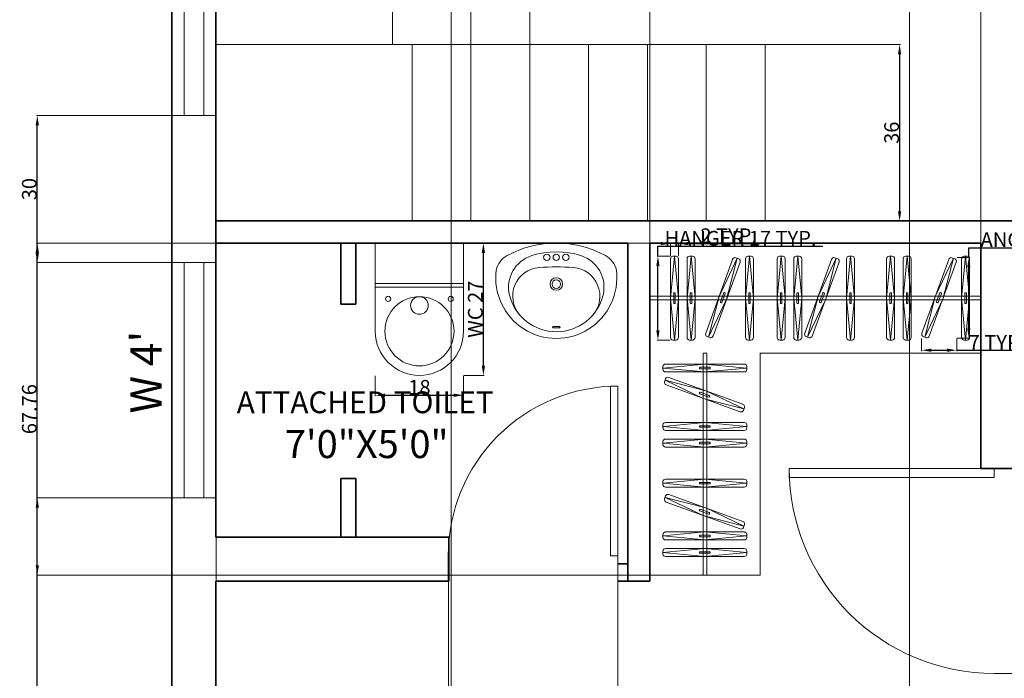
# Model space of a CAD drawing. Units: feet. Extents: x -297 to 770, y -228 to 625.
# Tile 2 of 14: x 351 to 552, y -40 to 95. Entities that reach past the tile are written whole.
import ezdxf

# ---------------------------------------------------------------- set-up
doc = ezdxf.new("R2010")
doc.units = ezdxf.units.FT
doc.header["$MEASUREMENT"] = 0
for name, color, linetype, lineweight in [('A-ANNO-DIMS', 2, 'Continuous', 18), ('A-ANNO-TEXT', 7, 'Continuous', 18), ('A-AREA-IDEN', 7, 'Continuous', 25), ('A-FLOR-CASE', 8, 'Continuous', 18), ('A-FLOR-FIXT', 8, 'Continuous', 18), ('A-FLOR-STRS', 7, 'Continuous', 18), ('A-WALL', 7, 'Continuous', 35), ('doors', 30, 'Continuous', 18), ('Washbasin-detail', 251, 'Continuous', 13), ('Washbasin-outline', 250, 'Continuous', 18), ('windows', 30, 'Continuous', 18)]:
    doc.layers.add(name, color=color, linetype=linetype, lineweight=lineweight)
doc.styles.add('Annotative', font='arial.ttf')
doc.styles.get("Standard").update_dxf_attribs({"font": 'arial.ttf'})
doc.dimstyles.get("Standard").update_dxf_attribs({"dimtxt": 3, "dimasz": 2, "dimexe": 0.18, "dimexo": 0.0625, "dimgap": 0.09, "dimtad": 1, "dimtoh": 1, "dimdec": 1, "dimzin": 0, "dimdsep": 46, "dimlunit": 3, "dimtxsty": 'Standard', "dimcen": 0, "dimclre": 256, "dimadec": 0, "dimazin": 0, "dimtfac": 1, "dimtdec": 1, "dimtofl": 0, "dimtmove": 0, "dimatfit": 3, "dimfxl": 1, "dimtolj": 1, "dimtzin": 0, "dimlwe": -1, "dimarcsym": 0})

# ---------------------------------------------------------------- blocks, each defined once
blk = doc.blocks.new('*U4')
for p, q in [((0, 0), (0, 6)), ((40, 0), (40, 6))]:
    blk.add_line(p, q)
blk.add_lwpolyline([(0, 0), (0, -40), (1.75, -40), (1.75, 0)], close=True)
blk.add_arc((0, 0), 40, 270, 0)
blk = doc.blocks.new('A$C391A2D23')
for p, q in [((0, 0.75), (0, 0.5)), ((0.5, 0.75), (0, 0.75)), ((0.5, 0.5), (0.5, 0.75)), ((0.5, 0.52), (0, 0.52)), ((0, 0.25), (0, 0.5)), ((0, 0.5), (0.5, 0.5)), ((0.5, 0.25), (0.5, 0.5))]:
    blk.add_line(p, q)
for centre, radius in [((0.0726, 0.4337), 0.0146), ((0.4274, 0.4337), 0.0146), ((0.25, 0.25), 0.196), ((0.25, 0.396), 0.05)]:
    blk.add_circle(centre, radius)
blk.add_arc((0.25, 0.25), 0.25, 180, 0)
blk = doc.blocks.new('WIN-5FT')
for p, q in [((60, 6.5), (0, 6.5)), ((60, 2.5), (0, 2.5))]:
    blk.add_line(p, q)
blk.add_lwpolyline([(60, 0), (60, 9), (0, 9), (0, 0)], close=True)
blk = doc.blocks.new('WIN-4FT')
for p, q in [((48, 9), (0, 9)), ((0, 9), (0, 0)), ((48, 0), (48, 9)), ((0, 6.5), (48, 6.5)), ((0, 2.5), (48, 2.5)), ((0, 0), (48, 0))]:
    blk.add_line(p, q)
blk = doc.blocks.new('CLOTHES-HANGER')
for p, q in [((0.81, 17.12), (0, 8.56)), ((0, 16.57), (0, 0.55)), ((1.13, 17.12), (0.49, 17.12)), ((0.81, 17.12), (1.62, 8.56)), ((1.62, 16.57), (1.62, 0.55)), ((0.81, 0), (0, 8.56)), ((0.65, 9.54), (0.65, 7.57)), ((0.87, 9.65), (0.74, 9.65)), ((0.81, 0), (1.62, 8.56)), ((0.97, 9.54), (0.97, 7.57)), ((0.87, 7.47), (0.74, 7.47)), ((1.13, 0), (0.49, 0))]:
    blk.add_line(p, q)
for centre, major_axis, start_param, end_param in [((0.49, 16.57), (0, 0.546), 0, 1.570796), ((1.13, 16.57), (0, 0.546), 4.712389, 6.283185), ((0.74, 9.54), (0, 0.109), 0, 1.570796), ((0.87, 9.54), (0, 0.109), -1.570796, 0), ((0.74, 7.57), (0, 0.109), 1.570796, 3.141593), ((0.87, 7.57), (0, 0.109), 3.141593, 4.712389), ((0.49, 0.55), (0, 0.546), 1.570796, 3.141593), ((1.13, 0.55), (0, 0.546), 3.141593, 4.712389)]:
    blk.add_ellipse(centre, major_axis=major_axis, ratio=0.888892, start_param=start_param, end_param=end_param)
blk = doc.blocks.new('CLOTHES-HANGER-ANGLED')
for p, q in [((6.46, 16.22), (2.78, 8.46)), ((6.46, 16.22), (4.3, 7.9)), ((6.77, 16.11), (6.16, 16.33)), ((5.52, 15.98), (0.04, 0.93)), ((7.04, 15.43), (1.56, 0.37)), ((0.61, 0.14), (2.78, 8.46)), ((3.72, 9.16), (3.05, 7.31)), ((4.03, 9.05), (3.35, 7.2)), ((3.97, 9.18), (3.85, 9.23)), ((0.61, 0.14), (4.3, 7.9)), ((3.22, 7.13), (3.1, 7.17)), ((0.91, 0.03), (0.31, 0.25))]:
    blk.add_line(p, q)
for centre, major_axis, start_param, end_param in [((5.97, 15.82), (0.187, 0.513), 0, 1.570796), ((6.58, 15.6), (0.187, 0.513), -1.570796, 0), ((3.81, 9.12), (0.037, 0.103), 0, 1.570796), ((3.93, 9.08), (0.037, 0.103), 4.712389, 6.283185), ((3.14, 7.28), (0.037, 0.103), 1.570796, 3.141593), ((3.26, 7.23), (0.037, 0.103), 3.141593, 4.712389), ((0.49, 0.76), (0.187, 0.513), 1.570796, 3.141593), ((1.1, 0.54), (0.187, 0.513), 3.141593, 4.712389)]:
    blk.add_ellipse(centre, major_axis=major_axis, ratio=0.888892, start_param=start_param, end_param=end_param)
blk = doc.blocks.new('*D35')
at = {"layer": 'A-ANNO-DIMS', "transparency": 16777216}
for p, q in [((441.72, 48.96), (445.89, 48.96)), ((441.72, 21.96), (445.89, 21.96))]:
    blk.add_line(p, q, dxfattribs=at)
at = {"layer": 'A-ANNO-DIMS', "color": 0, "lineweight": -2, "transparency": 16777216}
blk.add_line((445.71, 23.96), (445.71, 46.96), dxfattribs=at)
at = {"layer": 'A-ANNO-DIMS', "color": 0, "transparency": 16777216}
for points in [[(445.37, 46.96), (446.04, 46.96), (445.71, 48.96)], [(445.37, 23.96), (446.04, 23.96), (445.71, 21.96)]]:
    blk.add_solid(points, dxfattribs=at)
at = {"layer": 'Defpoints', "color": 0, "transparency": 16777216}
for p in [(441.66, 48.96), (445.71, 48.96), (441.66, 21.96)]:
    blk.add_point(p, dxfattribs=at)
at = {"layer": 'A-ANNO-DIMS', "color": 0, "transparency": 16777216, "insert": (444.06, 35.46), "char_height": 3, "attachment_point": 5, "rotation": 90}
blk.add_mtext('\\A1;WC 27', dxfattribs=at)
blk = doc.blocks.new('*D36')
at = {"layer": 'A-ANNO-DIMS', "transparency": 16777216}
for p, q in [((423.66, 21.9), (423.66, 17.73)), ((441.66, 21.9), (441.66, 17.73))]:
    blk.add_line(p, q, dxfattribs=at)
at = {"layer": 'A-ANNO-DIMS', "color": 0, "lineweight": -2, "transparency": 16777216}
blk.add_line((425.66, 17.91), (439.66, 17.91), dxfattribs=at)
at = {"layer": 'A-ANNO-DIMS', "color": 0, "transparency": 16777216}
for points in [[(425.66, 18.25), (425.66, 17.58), (423.66, 17.91)], [(439.66, 18.25), (439.66, 17.58), (441.66, 17.91)]]:
    blk.add_solid(points, dxfattribs=at)
at = {"layer": 'Defpoints', "color": 0, "transparency": 16777216}
for p in [(423.66, 21.96), (441.66, 21.96), (441.66, 17.91)]:
    blk.add_point(p, dxfattribs=at)
at = {"layer": 'A-ANNO-DIMS', "color": 0, "transparency": 16777216, "insert": (432.66, 19.53), "char_height": 3, "attachment_point": 5}
blk.add_mtext('\\A1;18', dxfattribs=at)
blk = doc.blocks.new('*D39')
at = {"layer": 'A-ANNO-DIMS', "color": 0, "lineweight": -2, "transparency": 16777216}
for p, q in [((481.31, 46.29), (481.31, 48.29)), ((481.31, 48.29), (514.93, 48.29)), ((481.31, 31.17), (481.31, 44.29))]:
    blk.add_line(p, q, dxfattribs=at)
at = {"layer": 'A-ANNO-DIMS', "transparency": 16777216}
for p, q in [((483.81, 46.29), (481.13, 46.29)), ((483.81, 29.17), (481.13, 29.17))]:
    blk.add_line(p, q, dxfattribs=at)
at = {"layer": 'A-ANNO-DIMS', "color": 0, "transparency": 16777216}
for points in [[(480.97, 44.29), (481.64, 44.29), (481.31, 46.29)], [(480.97, 31.17), (481.64, 31.17), (481.31, 29.17)]]:
    blk.add_solid(points, dxfattribs=at)
at = {"layer": 'Defpoints', "color": 0, "transparency": 16777216}
for p in [(481.31, 46.29), (483.87, 46.29), (483.87, 29.17)]:
    blk.add_point(p, dxfattribs=at)
at = {"layer": 'A-ANNO-DIMS', "color": 0, "transparency": 16777216, "insert": (498.16, 49.93), "char_height": 3, "attachment_point": 5}
blk.add_mtext('\\A1;HANGER 17 TYP.', dxfattribs=at)
blk = doc.blocks.new('*D40')
at = {"layer": 'A-ANNO-DIMS', "color": 0, "lineweight": -2, "transparency": 16777216}
for p, q in [((481.87, 48.86), (479.87, 48.86)), ((487.49, 48.86), (502, 48.86))]:
    blk.add_line(p, q, dxfattribs=at)
at = {"layer": 'A-ANNO-DIMS', "transparency": 16777216}
for p, q in [((483.87, 46.35), (483.87, 49.04)), ((485.49, 46.35), (485.49, 49.04))]:
    blk.add_line(p, q, dxfattribs=at)
at = {"layer": 'A-ANNO-DIMS', "color": 0, "transparency": 16777216}
for points in [[(481.87, 49.19), (481.87, 48.52), (483.87, 48.86)], [(487.49, 49.19), (487.49, 48.52), (485.49, 48.86)]]:
    blk.add_solid(points, dxfattribs=at)
at = {"layer": 'Defpoints', "color": 0, "transparency": 16777216}
for p in [(485.49, 48.86), (483.87, 46.29), (485.49, 46.29)]:
    blk.add_point(p, dxfattribs=at)
at = {"layer": 'A-ANNO-DIMS', "color": 0, "transparency": 16777216, "insert": (495.74, 50.45), "char_height": 3, "attachment_point": 5}
blk.add_mtext('\\A1;2 TYP.', dxfattribs=at)
blk = doc.blocks.new('*D41')
at = {"layer": 'A-ANNO-DIMS', "color": 0, "lineweight": -2, "transparency": 16777216}
for p, q in [((544.72, 46), (544.72, 48)), ((544.72, 48), (597.08, 48)), ((544.72, 31.56), (544.72, 44))]:
    blk.add_line(p, q, dxfattribs=at)
at = {"layer": 'A-ANNO-DIMS', "transparency": 16777216}
for p, q in [((542.32, 46), (544.9, 46)), ((542.32, 29.56), (544.9, 29.56))]:
    blk.add_line(p, q, dxfattribs=at)
at = {"layer": 'A-ANNO-DIMS', "color": 0, "transparency": 16777216}
for points in [[(544.39, 44), (545.05, 44), (544.72, 46)], [(544.39, 31.56), (545.05, 31.56), (544.72, 29.56)]]:
    blk.add_solid(points, dxfattribs=at)
at = {"layer": 'Defpoints', "color": 0, "transparency": 16777216}
for p in [(542.25, 46), (544.72, 46), (542.25, 29.56)]:
    blk.add_point(p, dxfattribs=at)
at = {"layer": 'A-ANNO-DIMS', "color": 0, "transparency": 16777216, "insert": (570.94, 49.64), "char_height": 3, "attachment_point": 5}
blk.add_mtext('\\A1;ANGLED HANGER 16 TYP.', dxfattribs=at)
blk = doc.blocks.new('*D42')
at = {"layer": 'A-ANNO-DIMS', "transparency": 16777216}
for p, q in [((535.1, 29.5), (535.1, 26.92)), ((542.25, 29.5), (542.25, 26.92))]:
    blk.add_line(p, q, dxfattribs=at)
at = {"layer": 'A-ANNO-DIMS', "color": 0, "lineweight": -2, "transparency": 16777216}
for p, q in [((537.1, 27.1), (540.25, 27.1)), ((542.25, 27.1), (556.68, 27.1))]:
    blk.add_line(p, q, dxfattribs=at)
at = {"layer": 'A-ANNO-DIMS', "color": 0, "transparency": 16777216}
for points in [[(537.1, 27.43), (537.1, 26.76), (535.1, 27.1)], [(540.25, 27.43), (540.25, 26.76), (542.25, 27.1)]]:
    blk.add_solid(points, dxfattribs=at)
at = {"layer": 'Defpoints', "color": 0, "transparency": 16777216}
for p in [(535.1, 29.56), (542.25, 29.56), (542.25, 27.1)]:
    blk.add_point(p, dxfattribs=at)
at = {"layer": 'A-ANNO-DIMS', "color": 0, "transparency": 16777216, "insert": (550.47, 28.69), "char_height": 3, "attachment_point": 5}
blk.add_mtext('\\A1;7 TYP.', dxfattribs=at)
blk = doc.blocks.new('*D52')
at = {"layer": 'A-ANNO-DIMS', "transparency": 16777216}
for p, q in [((382.09, 74.96), (354.53, 74.96)), ((382.09, 44.96), (354.53, 44.96))]:
    blk.add_line(p, q, dxfattribs=at)
at = {"layer": 'A-ANNO-DIMS', "color": 0, "lineweight": -2, "transparency": 16777216}
blk.add_line((354.71, 46.96), (354.71, 72.96), dxfattribs=at)
at = {"layer": 'A-ANNO-DIMS', "color": 0, "transparency": 16777216}
for points in [[(354.37, 72.96), (355.04, 72.96), (354.71, 74.96)], [(354.37, 46.96), (355.04, 46.96), (354.71, 44.96)]]:
    blk.add_solid(points, dxfattribs=at)
at = {"layer": 'Defpoints', "color": 0, "transparency": 16777216}
for p in [(354.71, 74.96), (382.16, 74.96), (382.16, 44.96)]:
    blk.add_point(p, dxfattribs=at)
at = {"layer": 'A-ANNO-DIMS', "color": 0, "transparency": 16777216, "insert": (353.08, 59.96), "char_height": 3, "attachment_point": 5, "rotation": 90}
blk.add_mtext('\\A1;30', dxfattribs=at)
blk = doc.blocks.new('*D53')
at = {"layer": 'A-ANNO-DIMS', "transparency": 16777216}
for p, q in [((382.09, -3.04), (354.53, -3.04)), ((382.09, -173.04), (354.53, -173.04))]:
    blk.add_line(p, q, dxfattribs=at)
at = {"layer": 'A-ANNO-DIMS', "color": 0, "lineweight": -2, "transparency": 16777216}
blk.add_line((354.71, -171.04), (354.71, -5.04), dxfattribs=at)
at = {"layer": 'A-ANNO-DIMS', "color": 0, "transparency": 16777216}
for points in [[(354.37, -5.04), (355.04, -5.04), (354.71, -3.04)], [(354.37, -171.04), (355.04, -171.04), (354.71, -173.04)]]:
    blk.add_solid(points, dxfattribs=at)
at = {"layer": 'Defpoints', "color": 0, "transparency": 16777216}
for p in [(354.71, -3.04), (382.16, -3.04), (382.16, -173.04)]:
    blk.add_point(p, dxfattribs=at)
at = {"layer": 'A-ANNO-DIMS', "color": 0, "transparency": 16777216, "insert": (353.08, -88.04), "char_height": 3, "attachment_point": 5, "rotation": 90}
blk.add_mtext('\\A1;170', dxfattribs=at)
blk = doc.blocks.new('*D57')
at = {"layer": 'A-ANNO-DIMS', "transparency": 16777216}
for p, q in [((391.16, -163.97), (391.16, 367.22)), ((439.16, -163.97), (439.16, 367.22))]:
    blk.add_line(p, q, dxfattribs=at)
at = {"layer": 'A-ANNO-DIMS', "color": 0, "lineweight": -2, "transparency": 16777216}
blk.add_line((393.16, 367.04), (437.16, 367.04), dxfattribs=at)
at = {"layer": 'A-ANNO-DIMS', "color": 0, "transparency": 16777216}
for points in [[(393.16, 367.38), (393.16, 366.71), (391.16, 367.04)], [(437.16, 367.38), (437.16, 366.71), (439.16, 367.04)]]:
    blk.add_solid(points, dxfattribs=at)
at = {"layer": 'Defpoints', "color": 0, "transparency": 16777216}
for p in [(439.16, 367.04), (391.16, -164.04), (439.16, -164.04)]:
    blk.add_point(p, dxfattribs=at)
at = {"layer": 'A-ANNO-DIMS', "color": 0, "transparency": 16777216, "insert": (415.16, 368.66), "char_height": 3, "attachment_point": 5}
blk.add_mtext('\\A1;48', dxfattribs=at)
blk = doc.blocks.new('*D67')
at = {"layer": 'A-ANNO-DIMS', "transparency": 16777216}
for p, q in [((532.66, 197.4), (532.66, -227.67)), ((561.66, 197.4), (561.66, -227.67))]:
    blk.add_line(p, q, dxfattribs=at)
at = {"layer": 'A-ANNO-DIMS', "color": 0, "lineweight": -2, "transparency": 16777216}
blk.add_line((534.66, -227.49), (559.66, -227.49), dxfattribs=at)
at = {"layer": 'A-ANNO-DIMS', "color": 0, "transparency": 16777216}
for points in [[(534.66, -227.15), (534.66, -227.82), (532.66, -227.49)], [(559.66, -227.15), (559.66, -227.82), (561.66, -227.49)]]:
    blk.add_solid(points, dxfattribs=at)
at = {"layer": 'Defpoints', "color": 0, "transparency": 16777216}
for p in [(532.66, 197.46), (561.66, 197.46), (561.66, -227.49)]:
    blk.add_point(p, dxfattribs=at)
at = {"layer": 'A-ANNO-DIMS', "color": 0, "transparency": 16777216, "insert": (547.16, -225.87), "char_height": 3, "attachment_point": 5}
blk.add_mtext('\\A1;29', dxfattribs=at)
blk = doc.blocks.new('*D69')
at = {"layer": 'A-ANNO-DIMS', "transparency": 16777216}
for p, q in [((438.62, -20.1), (438.62, -227.67)), ((473.16, -20.1), (473.16, -227.67))]:
    blk.add_line(p, q, dxfattribs=at)
at = {"layer": 'A-ANNO-DIMS', "color": 0, "lineweight": -2, "transparency": 16777216}
blk.add_line((440.62, -227.49), (471.16, -227.49), dxfattribs=at)
at = {"layer": 'A-ANNO-DIMS', "color": 0, "transparency": 16777216}
for points in [[(440.62, -227.15), (440.62, -227.82), (438.62, -227.49)], [(471.16, -227.15), (471.16, -227.82), (473.16, -227.49)]]:
    blk.add_solid(points, dxfattribs=at)
at = {"layer": 'Defpoints', "color": 0, "transparency": 16777216}
for p in [(438.62, -20.04), (473.16, -20.04), (473.16, -227.49)]:
    blk.add_point(p, dxfattribs=at)
at = {"layer": 'A-ANNO-DIMS', "color": 0, "transparency": 16777216, "insert": (455.89, -225.86), "char_height": 3, "attachment_point": 5}
blk.add_mtext('\\A1;34.53', dxfattribs=at)
blk = doc.blocks.new('*D72')
at = {"layer": 'A-ANNO-DIMS', "transparency": 16777216}
for p, q in [((479.66, 49.03), (479.66, 367.22)), ((547.16, 49.03), (547.16, 367.22))]:
    blk.add_line(p, q, dxfattribs=at)
at = {"layer": 'A-ANNO-DIMS', "color": 0, "lineweight": -2, "transparency": 16777216}
blk.add_line((481.66, 367.04), (545.16, 367.04), dxfattribs=at)
at = {"layer": 'A-ANNO-DIMS', "color": 0, "transparency": 16777216}
for points in [[(481.66, 367.38), (481.66, 366.71), (479.66, 367.04)], [(545.16, 367.38), (545.16, 366.71), (547.16, 367.04)]]:
    blk.add_solid(points, dxfattribs=at)
at = {"layer": 'Defpoints', "color": 0, "transparency": 16777216}
for p in [(547.16, 367.04), (479.66, 48.96), (547.16, 48.96)]:
    blk.add_point(p, dxfattribs=at)
at = {"layer": 'A-ANNO-DIMS', "color": 0, "transparency": 16777216, "insert": (513.41, 368.66), "char_height": 3, "attachment_point": 5}
blk.add_mtext('\\A1;67.5', dxfattribs=at)
blk = doc.blocks.new('*D73')
at = {"layer": 'A-ANNO-DIMS', "transparency": 16777216}
for p, q in [((479.59, 48.96), (354.53, 48.96)), ((479.59, -18.8), (354.53, -18.8))]:
    blk.add_line(p, q, dxfattribs=at)
at = {"layer": 'A-ANNO-DIMS', "color": 0, "lineweight": -2, "transparency": 16777216}
blk.add_line((354.71, -16.8), (354.71, 46.96), dxfattribs=at)
at = {"layer": 'A-ANNO-DIMS', "color": 0, "transparency": 16777216}
for points in [[(354.37, 46.96), (355.04, 46.96), (354.71, 48.96)], [(354.37, -16.8), (355.04, -16.8), (354.71, -18.8)]]:
    blk.add_solid(points, dxfattribs=at)
at = {"layer": 'Defpoints', "color": 0, "transparency": 16777216}
for p in [(354.71, 48.96), (479.66, 48.96), (479.66, -18.8)]:
    blk.add_point(p, dxfattribs=at)
at = {"layer": 'A-ANNO-DIMS', "color": 0, "transparency": 16777216, "insert": (353.08, 15.08), "char_height": 3, "attachment_point": 5, "rotation": 90}
blk.add_mtext('\\A1;67.76', dxfattribs=at)
blk = doc.blocks.new('*D76')
at = {"layer": 'A-ANNO-DIMS', "transparency": 16777216}
for p, q in [((443.16, 89.53), (443.16, 367.22)), ((455.16, 89.53), (455.16, 367.22))]:
    blk.add_line(p, q, dxfattribs=at)
at = {"layer": 'A-ANNO-DIMS', "color": 0, "lineweight": -2, "transparency": 16777216}
blk.add_line((445.16, 367.04), (453.16, 367.04), dxfattribs=at)
at = {"layer": 'A-ANNO-DIMS', "color": 0, "transparency": 16777216}
for points in [[(445.16, 367.38), (445.16, 366.71), (443.16, 367.04)], [(453.16, 367.38), (453.16, 366.71), (455.16, 367.04)]]:
    blk.add_solid(points, dxfattribs=at)
at = {"layer": 'Defpoints', "color": 0, "transparency": 16777216}
for p in [(455.16, 367.04), (443.16, 89.46), (455.16, 89.46)]:
    blk.add_point(p, dxfattribs=at)
at = {"layer": 'A-ANNO-DIMS', "color": 0, "transparency": 16777216, "insert": (449.16, 368.64), "char_height": 3, "attachment_point": 5}
blk.add_mtext('\\A1;12', dxfattribs=at)
blk = doc.blocks.new('*D77')
at = {"layer": 'A-ANNO-DIMS', "transparency": 16777216}
for p, q in [((503.22, 89.46), (530.79, 89.46)), ((503.22, 53.46), (530.79, 53.46))]:
    blk.add_line(p, q, dxfattribs=at)
at = {"layer": 'A-ANNO-DIMS', "color": 0, "lineweight": -2, "transparency": 16777216}
blk.add_line((530.61, 87.46), (530.61, 55.46), dxfattribs=at)
at = {"layer": 'A-ANNO-DIMS', "color": 0, "transparency": 16777216}
for points in [[(530.27, 87.46), (530.94, 87.46), (530.61, 89.46)], [(530.27, 55.46), (530.94, 55.46), (530.61, 53.46)]]:
    blk.add_solid(points, dxfattribs=at)
at = {"layer": 'Defpoints', "color": 0, "transparency": 16777216}
for p in [(503.16, 89.46), (503.16, 53.46), (530.61, 53.46)]:
    blk.add_point(p, dxfattribs=at)
at = {"layer": 'A-ANNO-DIMS', "color": 0, "transparency": 16777216, "insert": (528.98, 71.46), "char_height": 3, "attachment_point": 5, "rotation": 90}
blk.add_mtext('\\A1;36', dxfattribs=at)

msp = doc.modelspace()

# ---------------------------------------------------------------- linework, layer by layer
at = {"layer": 'A-FLOR-CASE'}
for p, q in [((479.655, 48.963), (547.094, 48.963)), ((479.655, 26.483), (479.655, 48.963)), ((479.655, 48.963), (547.094, 48.963)), ((479.655, 26.483), (479.655, 48.963)), ((479.655, 48.963), (547.094, 48.963)), ((479.655, 26.483), (479.655, 48.963)), ((547.094, 26.483), (547.094, 48.963)), ((547.094, 26.483), (547.094, 48.963)), ((547.094, 26.483), (547.094, 48.963)), ((479.655, 38.098), (547.094, 38.098)), ((479.655, 38.098), (547.094, 38.098)), ((479.655, 38.098), (547.094, 38.098)), ((479.655, 37.348), (547.094, 37.348)), ((479.655, 37.348), (547.094, 37.348)), ((479.655, 37.348), (547.094, 37.348)), ((479.655, -18.797), (479.655, 26.483)), ((490.52, 26.483), (491.27, 26.483)), ((490.52, 26.483), (491.27, 26.483)), ((490.52, 26.483), (491.27, 26.483)), ((491.27, 26.483), (490.52, 26.483)), ((490.52, -18.797), (490.52, 26.483)), ((491.27, -18.797), (491.27, 26.483)), ((502.135, -18.797), (502.135, 26.483)), ((502.135, 26.483), (547.094, 26.483)), ((479.655, -18.797), (502.135, -18.797))]:
    msp.add_line(p, q, dxfattribs=at)
at = {"layer": 'A-FLOR-STRS'}
for p, q in [((427.155, 89.463), (427.155, 173.463)), ((503.155, 89.463), (391.155, 89.463)), ((431.155, 53.463), (431.155, 89.463)), ((443.155, 53.463), (443.155, 89.463)), ((455.155, 53.463), (455.155, 89.463)), ((467.155, 53.463), (467.155, 89.463)), ((479.155, 53.463), (479.155, 89.463)), ((491.155, 53.463), (491.155, 89.463)), ((503.155, 53.463), (503.155, 89.463))]:
    msp.add_line(p, q, dxfattribs=at)
at = {"layer": 'A-WALL'}
for p, q in [((391.155, 53.463), (556.155, 53.463)), ((391.155, 48.963), (475.155, 48.963)), ((416.655, 36.463), (416.655, 48.963)), ((419.655, 36.463), (419.655, 48.963)), ((475.155, 48.963), (475.155, -20.037)), ((479.655, 48.963), (479.655, -20.037)), ((479.655, 48.963), (547.155, 48.963)), ((547.155, 2.963), (547.155, 48.963)), ((416.655, 36.463), (419.655, 36.463)), ((547.155, 2.963), (556.155, 2.963)), ((416.655, -11.037), (416.655, 0.963)), ((416.655, 0.963), (419.655, 0.963)), ((419.655, -11.037), (419.655, 0.963)), ((438.624, -11.037), (391.155, -11.037)), ((438.624, -20.037), (438.624, -11.037)), ((473.155, -16.453), (475.155, -16.453)), ((391.155, -20.037), (391.155, -164.037)), ((438.624, -20.037), (391.155, -20.037)), ((473.155, -20.041), (475.655, -20.037)), ((479.655, -20.037), (475.155, -20.037))]:
    msp.add_line(p, q, dxfattribs=at)
for points in [[(685.155, 306.963), (382.155, 306.963), (382.155, -173.037), (556.155, -173.037)], [(391.155, 173.463), (391.155, -11.037)]]:
    msp.add_lwpolyline(points, dxfattribs=at)
at = {"layer": 'Washbasin-detail'}
for p, q in [((459.943, 31.957), (460.577, 31.957)), ((459.943, 31.667), (460.577, 31.667)), ((461.211, 31.957), (460.577, 31.957)), ((461.211, 31.667), (460.577, 31.667))]:
    msp.add_line(p, q, dxfattribs=at)
for centre, radius in [((458.631, 46.044), 0.662), ((460.577, 46.044), 0.662), ((462.523, 46.044), 0.662), ((460.577, 40.595), 1.265), ((460.577, 40.595), 0.876)]:
    msp.add_circle(centre, radius, dxfattribs=at)
for centre, radius, start, end in [((457.543, 38.121), 5.856, 94.57625, 220.13804), ((460.577, 0.216), 43.882, 85.42376, 94.57625), ((463.611, 38.121), 5.856, 319.86196, 85.42376), ((459.943, 31.812), 0.145, 90, 270), ((461.211, 31.812), 0.145, 270, 90)]:
    msp.add_arc(centre, radius, start, end, dxfattribs=at)
at = {"layer": 'Washbasin-outline'}
for centre, radius, start, end in [((460.577, 28.132), 20.831, 61.20636, 118.79365), ((452.713, 42.44), 4.504, 118.79365, 167.11194), ((457.598, 39.947), 6.757, 107.43481, 193.79872), ((460.577, 30.461), 16.7, 72.56519, 107.43481), ((463.556, 39.947), 6.757, 346.20128, 72.56519), ((468.441, 42.44), 4.504, 12.88807, 61.20636), ((460.577, 41.86), 12.357, 172.63359, 7.36642), ((460.577, 40.679), 9.824, 193.79872, 346.20128)]:
    msp.add_arc(centre, radius, start, end, dxfattribs=at)

# ---------------------------------------------------------------- block references
at = {"layer": 'A-FLOR-CASE'}
for name, p in [('CLOTHES-HANGER', (483.874, 29.174)), ('CLOTHES-HANGER', (483.874, 29.174)), ('CLOTHES-HANGER', (483.874, 29.174)), ('CLOTHES-HANGER', (487.259, 29.174)), ('CLOTHES-HANGER', (487.259, 29.174)), ('CLOTHES-HANGER', (487.259, 29.174)), ('CLOTHES-HANGER', (499.18, 29.174)), ('CLOTHES-HANGER', (499.18, 29.174)), ('CLOTHES-HANGER', (499.18, 29.174)), ('CLOTHES-HANGER', (505.631, 29.174)), ('CLOTHES-HANGER', (505.631, 29.174)), ('CLOTHES-HANGER', (505.631, 29.174)), ('CLOTHES-HANGER', (509.016, 29.174)), ('CLOTHES-HANGER', (509.016, 29.174)), ('CLOTHES-HANGER', (509.016, 29.174)), ('CLOTHES-HANGER', (519.787, 29.174)), ('CLOTHES-HANGER', (519.787, 29.174)), ('CLOTHES-HANGER', (519.787, 29.174)), ('CLOTHES-HANGER', (527.961, 29.174)), ('CLOTHES-HANGER', (527.961, 29.174)), ('CLOTHES-HANGER', (527.961, 29.174)), ('CLOTHES-HANGER', (531.346, 29.174)), ('CLOTHES-HANGER', (531.346, 29.174)), ('CLOTHES-HANGER', (531.346, 29.174)), ('CLOTHES-HANGER', (543.266, 29.174)), ('CLOTHES-HANGER', (543.266, 29.174)), ('CLOTHES-HANGER', (543.266, 29.174)), ('CLOTHES-HANGER-ANGLED', (491.026, 29.628)), ('CLOTHES-HANGER-ANGLED', (491.026, 29.628)), ('CLOTHES-HANGER-ANGLED', (491.026, 29.628)), ('CLOTHES-HANGER-ANGLED', (511.229, 29.628)), ('CLOTHES-HANGER-ANGLED', (511.229, 29.628)), ('CLOTHES-HANGER-ANGLED', (511.229, 29.628)), ('CLOTHES-HANGER-ANGLED', (535.112, 29.628)), ('CLOTHES-HANGER-ANGLED', (535.112, 29.628)), ('CLOTHES-HANGER-ANGLED', (535.112, 29.628))]:
    msp.add_blockref(name, p, dxfattribs=at)
for name, p, rotation in [('CLOTHES-HANGER', (499.444, 22.656), 90.00000000745611), ('CLOTHES-HANGER-ANGLED', (498.99, 14.502), 90.00000000756445), ('CLOTHES-HANGER', (499.444, 10.735), 89.99999999975248), ('CLOTHES-HANGER', (499.444, 7.35), 90.00000000664404), ('CLOTHES-HANGER', (499.444, -0.824), 89.99999999245442), ('CLOTHES-HANGER-ANGLED', (498.99, -9.381), 90.00000000147148), ('CLOTHES-HANGER', (499.444, -11.595), 89.99999999529221), ('CLOTHES-HANGER', (499.444, -14.98), 89.9999999888058)]:
    msp.add_blockref(name, p, dxfattribs=dict(at, rotation=rotation))
at = {"layer": 'A-FLOR-FIXT', "xscale": 36, "yscale": 36, "zscale": 36}
msp.add_blockref('A$C391A2D23', (423.655, 21.963), dxfattribs=at)
at = {"layer": 'doors'}
for p, xscale, yscale, zscale, rotation in [((473.155, -14.85), 0.865479532060625, 0.865479532060625, 0.865479532060625, 180), ((549.888, 2.963), 1.044609893629039, 1.044609893629039, 1.044609893629039, 270)]:
    msp.add_blockref('*U4', p, dxfattribs=dict(at, xscale=xscale, yscale=yscale, zscale=zscale, rotation=rotation))
at = {"layer": 'windows'}
for name, p, rotation in [('WIN-5FT', (391.155, 74.963), 90.00000000000003), ('WIN-4FT', (391.155, -3.037), 89.99999999999987)]:
    msp.add_blockref(name, p, dxfattribs=dict(at, rotation=rotation))

# ---------------------------------------------------------------- texts
at = {"layer": 'A-ANNO-TEXT', "style": 'Annotative'}
msp.add_text("W 4'", height=6.4048, rotation=90, dxfattribs=at).set_placement((380.073, 14.185))
at = {"layer": 'A-AREA-IDEN', "style": 'Annotative'}
for s, height, p in [('ATTACHED TOILET', 4.44341, (395.382, 14.251)), ('7\'0"X5\'0"', 5.696, (405.209, 5.101))]:
    msp.add_text(s, height=height, dxfattribs=at).set_placement(p)

# ---------------------------------------------------------------- dimensions: what is measured, and where the dimension line sits
at = {"layer": 'A-ANNO-DIMS'}
for base, p1, p2, override, picture, middle in [((439.155, 367.042), (391.155, -164.037), (439.155, -164.037), {"dimdec": 0, "dimlfac": 1, "dimrnd": 0, "dimzin": 0, "dimdsep": 46, "dimlunit": 2}, '*D57', (415.155, 368.664)), ((455.155, 367.042), (443.155, 89.463), (455.155, 89.463), {"dimdec": 0, "dimlfac": 1, "dimrnd": 0, "dimzin": 0, "dimdsep": 46, "dimlunit": 2}, '*D76', (449.155, 368.638)), ((547.155, 367.042), (479.655, 48.963), (547.155, 48.963), {"dimdec": 1, "dimlfac": 1, "dimrnd": 0, "dimzin": 0, "dimdsep": 46, "dimlunit": 2}, '*D72', (513.405, 368.664)), ((561.655, -227.487), (532.655, 197.463), (561.655, 197.463), {"dimdec": 0, "dimlfac": 1, "dimrnd": 0, "dimzin": 0, "dimdsep": 46, "dimlunit": 2}, '*D67', (547.155, -225.866)), ((441.655, 17.913), (423.655, 21.963), (441.655, 21.963), {"dimdec": 0, "dimlfac": 1, "dimrnd": 0, "dimzin": 0, "dimdsep": 46, "dimlunit": 2}, '*D36', (432.655, 19.534)), ((473.155, -227.487), (438.624, -20.037), (473.155, -20.041), {"dimdec": 2, "dimlfac": 1, "dimrnd": 0, "dimzin": 0, "dimdsep": 46, "dimlunit": 2}, '*D69', (455.889, -225.865))]:
    dim = msp.add_linear_dim(base=base, p1=p1, p2=p2, dimstyle='Standard', override=override, dxfattribs=at)
    dim.commit()
    dim.dimension.update_dxf_attribs({"geometry": picture, "text_midpoint": middle})
for base, p1, p2, angle, override, picture, middle in [((530.605, 53.463), (503.155, 89.463), (503.155, 53.463), 270, {"dimdec": 0, "dimlfac": 1, "dimrnd": 0, "dimzin": 0, "dimdsep": 46, "dimlunit": 2}, '*D77', (528.983, 71.463)), ((354.705, 74.963), (382.155, 44.963), (382.155, 74.963), 90, {"dimdec": 0, "dimlfac": 1, "dimrnd": 0, "dimzin": 0, "dimdsep": 46, "dimlunit": 2}, '*D52', (353.083, 59.963)), ((354.705, 48.963), (479.655, -18.797), (479.655, 48.963), 90, {"dimdec": 2, "dimlfac": 1, "dimrnd": 0, "dimzin": 0, "dimdsep": 46, "dimlunit": 2}, '*D73', (353.084, 15.083)), ((354.705, -3.037), (382.155, -173.037), (382.155, -3.037), 90, {"dimdec": 0, "dimlfac": 1, "dimrnd": 0, "dimzin": 0, "dimdsep": 46, "dimlunit": 2}, '*D53', (353.084, -88.037))]:
    dim = msp.add_linear_dim(base=base, p1=p1, p2=p2, angle=angle, dimstyle='Standard', override=override, dxfattribs=at)
    dim.commit()
    dim.dimension.update_dxf_attribs({"geometry": picture, "text_midpoint": middle})
for base, p1, p2, text, picture, middle in [((544.719, 46.003), (542.253, 29.562), (542.253, 46.003), 'ANGLED HANGER <> TYP.', '*D41', (570.945, 49.644)), ((481.307, 46.29), (483.874, 29.174), (483.874, 46.29), 'HANGER <> TYP.', '*D39', (498.165, 49.931)), ((445.705, 48.963), (441.655, 21.963), (441.655, 48.963), 'WC <>', '*D35', (444.064, 35.463))]:
    dim = msp.add_linear_dim(base=base, p1=p1, p2=p2, angle=90, text=text, dimstyle='Standard', override={"dimdec": 0, "dimlfac": 1, "dimrnd": 0, "dimzin": 0, "dimdsep": 46, "dimlunit": 2}, dxfattribs=at)
    dim.commit()
    dim.dimension.update_dxf_attribs({"geometry": picture, "text_midpoint": middle})
for base, p1, p2, picture, middle in [((485.493, 48.857), (483.874, 46.29), (485.493, 46.29), '*D40', (495.744, 50.455)), ((542.253, 27.096), (535.099, 29.562), (542.253, 29.562), '*D42', (550.467, 28.687))]:
    dim = msp.add_linear_dim(base=base, p1=p1, p2=p2, text='<> TYP.', dimstyle='Standard', override={"dimdec": 0, "dimlfac": 1, "dimrnd": 0, "dimzin": 0, "dimdsep": 46, "dimlunit": 2}, dxfattribs=at)
    dim.commit()
    dim.dimension.update_dxf_attribs({"geometry": picture, "text_midpoint": middle})

doc.saveas('drawing.dxf')
